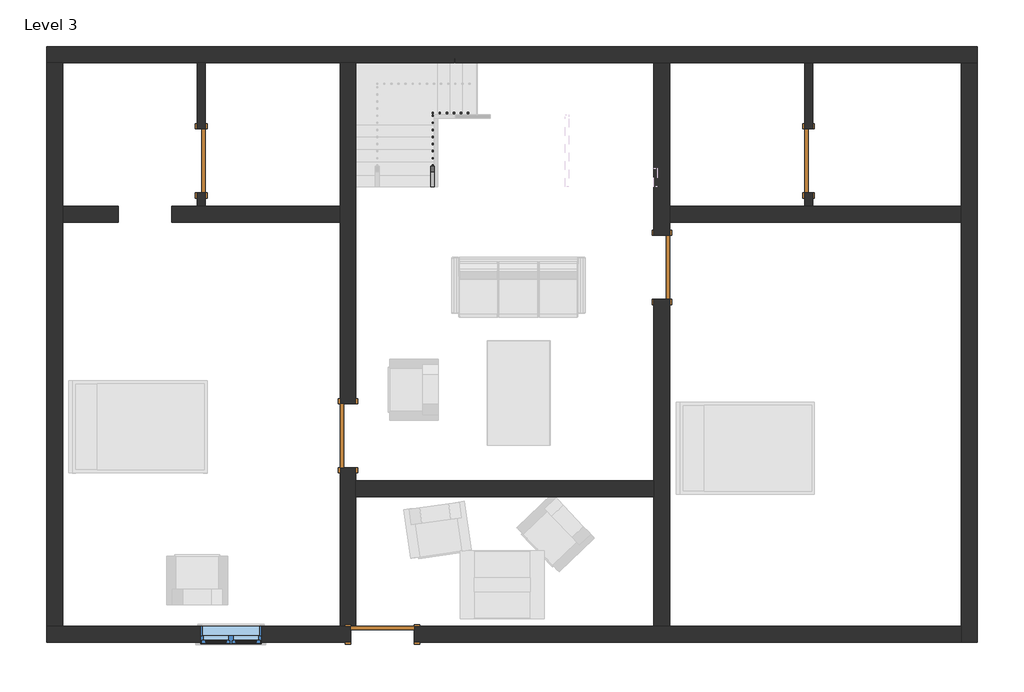
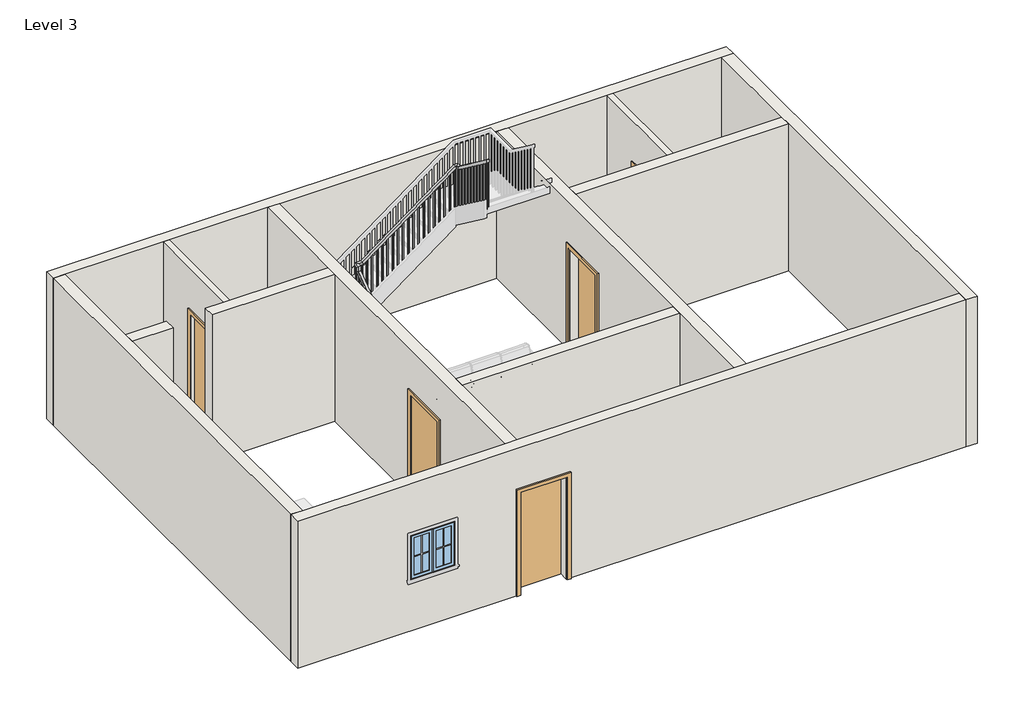
# One storey, part 1 of 2: 12 walls, 5 doors, 1 railing, 1 window.
"""IFC4 building model written with IfcOpenShell, lengths in millimetres."""

from ifc_helpers import new_model, si_unit, frame, origin, place, context, project, spatial, polyline, outline, extrude, faceted_brep, transform, mapped, element, save
from components import door_e5f9f3c4, door_a90ba1ad, door_305aa2a5, window_339605e1

model = new_model("IFC4")

# Units and contexts
model_context = context("Model", 3, world=origin())
ifc_project = project(units=[si_unit("LENGTHUNIT", "METRE", prefix="MILLI")], contexts=[model_context])

# Site, building, storey
site = spatial("IfcSite", under=ifc_project)
building = spatial("IfcBuilding", under=site)
storey = spatial("IfcBuildingStorey", under=building, Name="Level 3", Elevation=3200.4)

# Doors
placement = place(None, origin())
door_shape = door_e5f9f3c4(model_context)
element("IfcDoor", 1, ObjectType="Single-Flush : 36\" x 84\"", at=placement, inside=storey, context=model_context, shape_type="MappedRepresentation", body=[
    mapped(door_shape, transform((-5709.1546642, 5087.2167606, 3200.4), x_axis=(0.0, -1.0, 0.0), y_axis=(1.0, 0.0, 0.0), z_axis=(0.0, 0.0, 1.0))),
])
door_2_shape = door_a90ba1ad(model_context)
element("IfcDoor", 2, ObjectType="Single-Flush : 36\" x 84\"", at=placement, inside=storey, context=model_context, shape_type="MappedRepresentation", body=[
    mapped(door_2_shape, transform((-3607.3046642, 1150.2167606, 3200.4), x_axis=(0.0, -1.0, 0.0), y_axis=(1.0, 0.0, 0.0), z_axis=(0.0, 0.0, 1.0))),
])
element("IfcDoor", 3, ObjectType="Single-Flush : 36\" x 84\"", at=placement, inside=storey, context=model_context, shape_type="MappedRepresentation", body=[
    mapped(door_2_shape, transform((888.4953358, 3563.2167606, 3200.4), x_axis=(0.0, 1.0, 0.0), y_axis=(-1.0, 0.0, 0.0), z_axis=(0.0, 0.0, 1.0))),
])
element("IfcDoor", 4, ObjectType="Single-Flush : 36\" x 84\"", at=placement, inside=storey, context=model_context, shape_type="MappedRepresentation", body=[
    mapped(door_2_shape, transform((-3112.0046642, -1694.5832394, 3200.4), x_axis=(-1.0, 0.0, 0.0), y_axis=(0.0, -1.0, 0.0), z_axis=(0.0, 0.0, 1.0))),
])
door_3_shape = door_305aa2a5(model_context)
element("IfcDoor", 5, ObjectType="Single-Flush : 36\" x 84\"", at=placement, inside=storey, context=model_context, shape_type="MappedRepresentation", body=[
    mapped(door_3_shape, transform((2990.3453358, 5087.2167606, 3200.4), x_axis=(0.0, -1.0, 0.0), y_axis=(1.0, 0.0, 0.0), z_axis=(0.0, 0.0, 1.0))),
])

# Railing
element("IfcRailing", 6, ObjectType="Handrail - Rectangular", at=placement, inside=storey, context=model_context, shape_type="SolidModel", body=[
    faceted_brep([(-2419.4972892, 4718.9167606, 4247.3217391), (-2419.4972892, 4718.9167606, 4183.9634439), (-2368.6972892, 4718.9167606, 4183.9634439), (-2368.6972892, 4718.9167606, 4247.3217391), (-2419.4972892, 5670.3536537, 4956.4672495), (-2419.4972892, 5721.1536537, 4930.9723083), (-2368.6972892, 5721.1536537, 4930.9723083), (-2368.6972892, 5670.3536537, 4956.4672495), (-2419.4972892, 5670.3536537, 5063.2733611), (-2419.4972892, 5721.1536537, 5012.4733611), (-2368.6972892, 5721.1536537, 5012.4733611), (-2368.6972892, 5670.3536537, 5063.2733611), (-2419.4972892, 5797.3536537, 5063.2733611), (-2419.4972892, 5797.3536537, 5012.4733611), (-2368.6972892, 5746.5536537, 5012.4733611), (-2368.6972892, 5746.5536537, 5063.2733611), (-2292.4972892, 5797.3536537, 5063.2733611), (-2275.6482431, 5797.3536537, 5012.4733611), (-2275.6482431, 5746.5536537, 5012.4733611), (-2292.4972892, 5746.5536537, 5063.2733611), (-474.1369697, 5797.3536537, 6418.5729781), (-457.2879235, 5797.3536537, 6367.7729781), (-457.2879235, 5746.5536537, 6367.7729781), (-474.1369697, 5746.5536537, 6418.5729781), (-394.2046642, 5797.3536537, 6418.5729781), (-394.2046642, 5797.3536537, 6367.7729781), (-445.0046642, 5746.5536537, 6367.7729781), (-445.0046642, 5746.5536537, 6418.5729781), (-394.2046642, 5717.4213483, 6418.5729781), (-394.2046642, 5700.5723021, 6367.7729781), (-445.0046642, 5700.5723021, 6367.7729781), (-445.0046642, 5717.4213483, 6418.5729781), (-394.2046642, 4718.9167606, 7162.8), (-445.0046642, 4718.9167606, 7162.8), (-445.0046642, 4718.9167606, 7099.4417047), (-394.2046642, 4718.9167606, 7099.4417047)], [[[0, 1, 2, 3]], [[1, 0, 4, 5]], [[2, 1, 5, 6]], [[3, 2, 6, 7]], [[0, 3, 7, 4]], [[5, 4, 8, 9]], [[6, 5, 9, 10]], [[7, 6, 10, 11]], [[4, 7, 11, 8]], [[9, 8, 12, 13]], [[10, 9, 13, 14]], [[11, 10, 14, 15]], [[8, 11, 15, 12]], [[13, 12, 16, 17]], [[14, 13, 17, 18]], [[15, 14, 18, 19]], [[12, 15, 19, 16]], [[17, 16, 20, 21]], [[18, 17, 21, 22]], [[19, 18, 22, 23]], [[16, 19, 23, 20]], [[21, 20, 24, 25]], [[22, 21, 25, 26]], [[23, 22, 26, 27]], [[20, 23, 27, 24]], [[25, 24, 28, 29]], [[26, 25, 29, 30]], [[27, 26, 30, 31]], [[24, 27, 31, 28]], [[32, 33, 34, 35]], [[29, 28, 32, 35]], [[30, 29, 35, 34]], [[31, 30, 34, 33]], [[28, 31, 33, 32]]]),
    extrude(outline(polyline([(4746.4286537, 7078.9359459), (4765.4786537, 7064.7371882), (4765.4786537, 6115.8782609), (4746.4286537, 6115.8782609), (4746.4286537, 7078.9359459)])), frame((-429.1296642, 0.0, 0.0), z_axis=(1.0, 0.0, 0.0), x_axis=(0.0, 1.0, 0.0)), (0.0, 0.0, 1.0), 19.05),
    extrude(outline(polyline([(4848.0286537, 7003.2092378), (4867.0786537, 6989.0104801), (4867.0786537, 6115.8782609), (4848.0286537, 6115.8782609), (4848.0286537, 7003.2092378)])), frame((-429.1296642, 0.0, 0.0), z_axis=(1.0, 0.0, 0.0), x_axis=(0.0, 1.0, 0.0)), (0.0, 0.0, 1.0), 19.05),
    extrude(outline(polyline([(4949.6286537, 6927.4825298), (4968.6786537, 6913.283772), (4968.6786537, 5983.3565217), (4949.6286537, 5983.3565217), (4949.6286537, 6927.4825298)])), frame((-429.1296642, 0.0, 0.0), z_axis=(1.0, 0.0, 0.0), x_axis=(0.0, 1.0, 0.0)), (0.0, 0.0, 1.0), 19.05),
    extrude(outline(polyline([(5051.2286537, 6851.7558217), (5070.2786537, 6837.5570639), (5070.2786537, 5983.3565217), (5051.2286537, 5983.3565217), (5051.2286537, 6851.7558217)])), frame((-429.1296642, 0.0, 0.0), z_axis=(1.0, 0.0, 0.0), x_axis=(0.0, 1.0, 0.0)), (0.0, 0.0, 1.0), 19.05),
    extrude(outline(polyline([(5152.8286537, 6776.0291136), (5171.8786537, 6761.8303559), (5171.8786537, 5850.8347826), (5152.8286537, 5850.8347826), (5152.8286537, 6776.0291136)])), frame((-429.1296642, 0.0, 0.0), z_axis=(1.0, 0.0, 0.0), x_axis=(0.0, 1.0, 0.0)), (0.0, 0.0, 1.0), 19.05),
    extrude(outline(polyline([(5254.4286537, 6700.3024055), (5273.4786537, 6686.1036478), (5273.4786537, 5718.3130435), (5254.4286537, 5718.3130435), (5254.4286537, 6700.3024055)])), frame((-429.1296642, 0.0, 0.0), z_axis=(1.0, 0.0, 0.0), x_axis=(0.0, 1.0, 0.0)), (0.0, 0.0, 1.0), 19.05),
    extrude(outline(polyline([(5356.0286537, 6624.5756975), (5375.0786537, 6610.3769397), (5375.0786537, 5718.3130435), (5356.0286537, 5718.3130435), (5356.0286537, 6624.5756975)])), frame((-429.1296642, 0.0, 0.0), z_axis=(1.0, 0.0, 0.0), x_axis=(0.0, 1.0, 0.0)), (0.0, 0.0, 1.0), 19.05),
    extrude(outline(polyline([(5457.6286537, 6548.8489894), (5476.6786537, 6534.6502316), (5476.6786537, 5585.7913043), (5457.6286537, 5585.7913043), (5457.6286537, 6548.8489894)])), frame((-429.1296642, 0.0, 0.0), z_axis=(1.0, 0.0, 0.0), x_axis=(0.0, 1.0, 0.0)), (0.0, 0.0, 1.0), 19.05),
    extrude(outline(polyline([(5559.2286537, 6473.1222813), (5578.2786537, 6458.9235236), (5578.2786537, 5585.7913043), (5559.2286537, 5585.7913043), (5559.2286537, 6473.1222813)])), frame((-429.1296642, 0.0, 0.0), z_axis=(1.0, 0.0, 0.0), x_axis=(0.0, 1.0, 0.0)), (0.0, 0.0, 1.0), 19.05),
    extrude(outline(polyline([(5660.8286537, 6397.3955732), (5679.8786537, 6383.1968155), (5679.8786537, 5453.2695652), (5660.8286537, 5453.2695652), (5660.8286537, 6397.3955732)])), frame((-429.1296642, 0.0, 0.0), z_axis=(1.0, 0.0, 0.0), x_axis=(0.0, 1.0, 0.0)), (0.0, 0.0, 1.0), 19.05),
    extrude(outline(polyline([(-473.2222892, 5762.4286537), (-473.2222892, 5781.4786537), (-454.1722892, 5781.4786537), (-454.1722892, 5762.4286537), (-473.2222892, 5762.4286537)])), frame((0.0, 0.0, 5453.2695652), z_axis=(0.0, 0.0, 1.0), x_axis=(1.0, 0.0, 0.0)), (0.0, 0.0, 1.0), 914.5034129),
    extrude(outline(polyline([(6294.3684819, -555.7722892), (6280.1697242, -574.8222892), (5320.7478261, -574.8222892), (5320.7478261, -555.7722892), (6294.3684819, -555.7722892)])), frame((0.0, 5762.4286537, 0.0), z_axis=(0.0, 1.0, 0.0), x_axis=(0.0, 0.0, 1.0)), (0.0, 0.0, 1.0), 19.05),
    extrude(outline(polyline([(6218.6417739, -657.3722892), (6204.4430161, -676.4222892), (5320.7478261, -676.4222892), (5320.7478261, -657.3722892), (6218.6417739, -657.3722892)])), frame((0.0, 5762.4286537, 0.0), z_axis=(0.0, 1.0, 0.0), x_axis=(0.0, 0.0, 1.0)), (0.0, 0.0, 1.0), 19.05),
    extrude(outline(polyline([(6142.9150658, -758.9722892), (6128.716308, -778.0222892), (5188.226087, -778.0222892), (5188.226087, -758.9722892), (6142.9150658, -758.9722892)])), frame((0.0, 5762.4286537, 0.0), z_axis=(0.0, 1.0, 0.0), x_axis=(0.0, 0.0, 1.0)), (0.0, 0.0, 1.0), 19.05),
    extrude(outline(polyline([(6067.1883577, -860.5722892), (6052.9896, -879.6222892), (5188.226087, -879.6222892), (5188.226087, -860.5722892), (6067.1883577, -860.5722892)])), frame((0.0, 5762.4286537, 0.0), z_axis=(0.0, 1.0, 0.0), x_axis=(0.0, 0.0, 1.0)), (0.0, 0.0, 1.0), 19.05),
    extrude(outline(polyline([(5991.4616496, -962.1722892), (5977.2628919, -981.2222892), (5055.7043478, -981.2222892), (5055.7043478, -962.1722892), (5991.4616496, -962.1722892)])), frame((0.0, 5762.4286537, 0.0), z_axis=(0.0, 1.0, 0.0), x_axis=(0.0, 0.0, 1.0)), (0.0, 0.0, 1.0), 19.05),
    extrude(outline(polyline([(5915.7349416, -1063.7722892), (5901.5361838, -1082.8222892), (5055.7043478, -1082.8222892), (5055.7043478, -1063.7722892), (5915.7349416, -1063.7722892)])), frame((0.0, 5762.4286537, 0.0), z_axis=(0.0, 1.0, 0.0), x_axis=(0.0, 0.0, 1.0)), (0.0, 0.0, 1.0), 19.05),
    extrude(outline(polyline([(5840.0082335, -1165.3722892), (5825.8094757, -1184.4222892), (4923.1826087, -1184.4222892), (4923.1826087, -1165.3722892), (5840.0082335, -1165.3722892)])), frame((0.0, 5762.4286537, 0.0), z_axis=(0.0, 1.0, 0.0), x_axis=(0.0, 0.0, 1.0)), (0.0, 0.0, 1.0), 19.05),
    extrude(outline(polyline([(5764.2815254, -1266.9722892), (5750.0827677, -1286.0222892), (4790.6608696, -1286.0222892), (4790.6608696, -1266.9722892), (5764.2815254, -1266.9722892)])), frame((0.0, 5762.4286537, 0.0), z_axis=(0.0, 1.0, 0.0), x_axis=(0.0, 0.0, 1.0)), (0.0, 0.0, 1.0), 19.05),
    extrude(outline(polyline([(5688.5548173, -1368.5722892), (5674.3560596, -1387.6222892), (4790.6608696, -1387.6222892), (4790.6608696, -1368.5722892), (5688.5548173, -1368.5722892)])), frame((0.0, 5762.4286537, 0.0), z_axis=(0.0, 1.0, 0.0), x_axis=(0.0, 0.0, 1.0)), (0.0, 0.0, 1.0), 19.05),
    extrude(outline(polyline([(5612.8281093, -1470.1722892), (5598.6293515, -1489.2222892), (4658.1391304, -1489.2222892), (4658.1391304, -1470.1722892), (5612.8281093, -1470.1722892)])), frame((0.0, 5762.4286537, 0.0), z_axis=(0.0, 1.0, 0.0), x_axis=(0.0, 0.0, 1.0)), (0.0, 0.0, 1.0), 19.05),
    extrude(outline(polyline([(5537.1014012, -1571.7722892), (5522.9026434, -1590.8222892), (4658.1391304, -1590.8222892), (4658.1391304, -1571.7722892), (5537.1014012, -1571.7722892)])), frame((0.0, 5762.4286537, 0.0), z_axis=(0.0, 1.0, 0.0), x_axis=(0.0, 0.0, 1.0)), (0.0, 0.0, 1.0), 19.05),
    extrude(outline(polyline([(5461.3746931, -1673.3722892), (5447.1759354, -1692.4222892), (4525.6173913, -1692.4222892), (4525.6173913, -1673.3722892), (5461.3746931, -1673.3722892)])), frame((0.0, 5762.4286537, 0.0), z_axis=(0.0, 1.0, 0.0), x_axis=(0.0, 0.0, 1.0)), (0.0, 0.0, 1.0), 19.05),
    extrude(outline(polyline([(5385.647985, -1774.9722892), (5371.4492273, -1794.0222892), (4525.6173913, -1794.0222892), (4525.6173913, -1774.9722892), (5385.647985, -1774.9722892)])), frame((0.0, 5762.4286537, 0.0), z_axis=(0.0, 1.0, 0.0), x_axis=(0.0, 0.0, 1.0)), (0.0, 0.0, 1.0), 19.05),
    extrude(outline(polyline([(5309.921277, -1876.5722892), (5295.7225192, -1895.6222892), (4393.0956522, -1895.6222892), (4393.0956522, -1876.5722892), (5309.921277, -1876.5722892)])), frame((0.0, 5762.4286537, 0.0), z_axis=(0.0, 1.0, 0.0), x_axis=(0.0, 0.0, 1.0)), (0.0, 0.0, 1.0), 19.05),
    extrude(outline(polyline([(5234.1945689, -1978.1722892), (5219.9958111, -1997.2222892), (4260.573913, -1997.2222892), (4260.573913, -1978.1722892), (5234.1945689, -1978.1722892)])), frame((0.0, 5762.4286537, 0.0), z_axis=(0.0, 1.0, 0.0), x_axis=(0.0, 0.0, 1.0)), (0.0, 0.0, 1.0), 19.05),
    extrude(outline(polyline([(5158.4678608, -2079.7722892), (5144.2691031, -2098.8222892), (4260.573913, -2098.8222892), (4260.573913, -2079.7722892), (5158.4678608, -2079.7722892)])), frame((0.0, 5762.4286537, 0.0), z_axis=(0.0, 1.0, 0.0), x_axis=(0.0, 0.0, 1.0)), (0.0, 0.0, 1.0), 19.05),
    extrude(outline(polyline([(5082.7411527, -2181.3722892), (5068.542395, -2200.4222892), (4128.0521739, -2200.4222892), (4128.0521739, -2181.3722892), (5082.7411527, -2181.3722892)])), frame((0.0, 5762.4286537, 0.0), z_axis=(0.0, 1.0, 0.0), x_axis=(0.0, 0.0, 1.0)), (0.0, 0.0, 1.0), 19.05),
    extrude(outline(polyline([(5007.0144447, -2282.9722892), (4992.8156869, -2302.0222892), (4128.0521739, -2302.0222892), (4128.0521739, -2282.9722892), (5007.0144447, -2282.9722892)])), frame((0.0, 5762.4286537, 0.0), z_axis=(0.0, 1.0, 0.0), x_axis=(0.0, 0.0, 1.0)), (0.0, 0.0, 1.0), 19.05),
    extrude(outline(polyline([(-2384.5722892, 5725.3917606), (-2403.6222892, 5725.3917606), (-2403.6222892, 5744.4417606), (-2384.5722892, 5744.4417606), (-2384.5722892, 5725.3917606)])), frame((0.0, 0.0, 3995.5304348), z_axis=(0.0, 0.0, 1.0), x_axis=(1.0, 0.0, 0.0)), (0.0, 0.0, 1.0), 1016.9429263),
    extrude(outline(polyline([(5623.7917606, 4858.4044377), (5642.8417606, 4872.6031954), (5642.8417606, 3995.5304348), (5623.7917606, 3995.5304348), (5623.7917606, 4858.4044377)])), frame((-2403.6222892, 0.0, 0.0), z_axis=(1.0, 0.0, 0.0), x_axis=(0.0, 1.0, 0.0)), (0.0, 0.0, 1.0), 19.05),
    extrude(outline(polyline([(5522.1917606, 4782.6777296), (5541.2417606, 4796.8764873), (5541.2417606, 3863.0086957), (5522.1917606, 3863.0086957), (5522.1917606, 4782.6777296)])), frame((-2403.6222892, 0.0, 0.0), z_axis=(1.0, 0.0, 0.0), x_axis=(0.0, 1.0, 0.0)), (0.0, 0.0, 1.0), 19.05),
    extrude(outline(polyline([(5420.5917606, 4706.9510215), (5439.6417606, 4721.1497793), (5439.6417606, 3863.0086957), (5420.5917606, 3863.0086957), (5420.5917606, 4706.9510215)])), frame((-2403.6222892, 0.0, 0.0), z_axis=(1.0, 0.0, 0.0), x_axis=(0.0, 1.0, 0.0)), (0.0, 0.0, 1.0), 19.05),
    extrude(outline(polyline([(5318.9917606, 4631.2243134), (5338.0417606, 4645.4230712), (5338.0417606, 3730.4869565), (5318.9917606, 3730.4869565), (5318.9917606, 4631.2243134)])), frame((-2403.6222892, 0.0, 0.0), z_axis=(1.0, 0.0, 0.0), x_axis=(0.0, 1.0, 0.0)), (0.0, 0.0, 1.0), 19.05),
    extrude(outline(polyline([(5217.3917606, 4555.4976054), (5236.4417606, 4569.6963631), (5236.4417606, 3597.9652174), (5217.3917606, 3597.9652174), (5217.3917606, 4555.4976054)])), frame((-2403.6222892, 0.0, 0.0), z_axis=(1.0, 0.0, 0.0), x_axis=(0.0, 1.0, 0.0)), (0.0, 0.0, 1.0), 19.05),
    extrude(outline(polyline([(5115.7917606, 4479.7708973), (5134.8417606, 4493.969655), (5134.8417606, 3597.9652174), (5115.7917606, 3597.9652174), (5115.7917606, 4479.7708973)])), frame((-2403.6222892, 0.0, 0.0), z_axis=(1.0, 0.0, 0.0), x_axis=(0.0, 1.0, 0.0)), (0.0, 0.0, 1.0), 19.05),
    extrude(outline(polyline([(5014.1917606, 4404.0441892), (5033.2417606, 4418.242947), (5033.2417606, 3465.4434783), (5014.1917606, 3465.4434783), (5014.1917606, 4404.0441892)])), frame((-2403.6222892, 0.0, 0.0), z_axis=(1.0, 0.0, 0.0), x_axis=(0.0, 1.0, 0.0)), (0.0, 0.0, 1.0), 19.05),
    extrude(outline(polyline([(4912.5917606, 4328.3174811), (4931.6417606, 4342.5162389), (4931.6417606, 3465.4434783), (4912.5917606, 3465.4434783), (4912.5917606, 4328.3174811)])), frame((-2403.6222892, 0.0, 0.0), z_axis=(1.0, 0.0, 0.0), x_axis=(0.0, 1.0, 0.0)), (0.0, 0.0, 1.0), 19.05),
    extrude(outline(polyline([(4810.9917606, 4252.5907731), (4830.0417606, 4266.7895308), (4830.0417606, 3332.9217391), (4810.9917606, 3332.9217391), (4810.9917606, 4252.5907731)])), frame((-2403.6222892, 0.0, 0.0), z_axis=(1.0, 0.0, 0.0), x_axis=(0.0, 1.0, 0.0)), (0.0, 0.0, 1.0), 19.05),
    extrude(outline(polyline([(-429.1296642, 5762.4286537), (-429.1296642, 5781.4786537), (-410.0796642, 5781.4786537), (-410.0796642, 5762.4286537), (-429.1296642, 5762.4286537)])), frame((0.0, 0.0, 5453.2695652), z_axis=(0.0, 0.0, 1.0), x_axis=(1.0, 0.0, 0.0)), (0.0, 0.0, 1.0), 914.5034129),
    extrude(outline(polyline([(-2384.5722892, 5762.4286537), (-2403.6222892, 5762.4286537), (-2403.6222892, 5781.4786537), (-2384.5722892, 5781.4786537), (-2384.5722892, 5762.4286537)])), frame((0.0, 0.0, 3995.5304348), z_axis=(0.0, 0.0, 1.0), x_axis=(1.0, 0.0, 0.0)), (0.0, 0.0, 1.0), 1016.9429263),
    extrude(outline(polyline([(4718.9167606, 7099.4417047), (4737.9667606, 7085.242947), (4737.9667606, 6115.8782609), (4718.9167606, 6115.8782609), (4718.9167606, 7099.4417047)])), frame((-429.1296642, 0.0, 0.0), z_axis=(1.0, 0.0, 0.0), x_axis=(0.0, 1.0, 0.0)), (0.0, 0.0, 1.0), 19.05),
    extrude(outline(polyline([(4718.9167606, 4183.9634439), (4737.9667606, 4198.1622016), (4737.9667606, 3332.9217391), (4718.9167606, 3332.9217391), (4718.9167606, 4183.9634439)])), frame((-2403.6222892, 0.0, 0.0), z_axis=(1.0, 0.0, 0.0), x_axis=(0.0, 1.0, 0.0)), (0.0, 0.0, 1.0), 19.05),
])

# Walls
element("IfcWall", 7, ObjectType="WALL4.5\"", at=placement, inside=storey, context=model_context, shape_type="SweptSolid", body=[
    extrude(outline(polyline([(4630.0167606, 5334.0), (4630.0167606, 3200.4), (4439.5167606, 3200.4), (4439.5167606, 6248.4), (6496.9167606, 6248.4), (6496.9167606, 3200.4), (5544.4167606, 3200.4), (5544.4167606, 5334.0), (4630.0167606, 5334.0)])), frame((-5766.3046642, 0.0, 0.0), z_axis=(1.0, 0.0, 0.0), x_axis=(0.0, 1.0, 0.0)), (0.0, 0.0, 1.0), 114.3),
])
element("IfcWall", 8, ObjectType="WALL4.5\"", at=placement, inside=storey, context=model_context, shape_type="SweptSolid", body=[
    extrude(outline(polyline([(4630.0167606, 5334.0), (4630.0167606, 3200.4), (4439.5167606, 3200.4), (4439.5167606, 6248.4), (6496.9167606, 6248.4), (6496.9167606, 3200.4), (5544.4167606, 3200.4), (5544.4167606, 5334.0), (4630.0167606, 5334.0)])), frame((2933.1953358, 0.0, 0.0), z_axis=(1.0, 0.0, 0.0), x_axis=(0.0, 1.0, 0.0)), (0.0, 0.0, 1.0), 114.3),
])
element("IfcWall", 9, ObjectType="WALL9\"", at=placement, inside=storey, context=model_context, shape_type="Brep", body=[
    faceted_brep([(-7925.3046642, 6496.9167606, 3200.4), (-7696.7046642, 6496.9167606, 3200.4), (-5766.3046642, 6496.9167606, 3200.4), (-5652.0046642, 6496.9167606, 3200.4), (-3721.6046642, 6496.9167606, 3200.4), (-3493.0046642, 6496.9167606, 3200.4), (774.1953358, 6496.9167606, 3200.4), (1002.7953358, 6496.9167606, 3200.4), (2933.1953358, 6496.9167606, 3200.4), (3047.4953358, 6496.9167606, 3200.4), (5181.0953358, 6496.9167606, 3200.4), (5409.6953358, 6496.9167606, 3200.4), (5409.6953358, 6496.9167606, 6248.4), (5181.0953358, 6496.9167606, 6248.4), (3047.4953358, 6496.9167606, 6248.4), (2933.1953358, 6496.9167606, 6248.4), (1002.7953358, 6496.9167606, 6248.4), (774.1953358, 6496.9167606, 6248.4), (-3493.0046642, 6496.9167606, 6248.4), (-3721.6046642, 6496.9167606, 6248.4), (-5652.0046642, 6496.9167606, 6248.4), (-5766.3046642, 6496.9167606, 6248.4), (-7696.7046642, 6496.9167606, 6248.4), (-7925.3046642, 6496.9167606, 6248.4), (-7925.3046642, 6725.5167606, 3200.4), (-7925.3046642, 6725.5167606, 6248.4), (5409.6953358, 6725.5167606, 6248.4), (5409.6953358, 6725.5167606, 3200.4)], [[[0, 1, 2, 3, 4, 5, 6, 7, 8, 9, 10, 11, 12, 13, 14, 15, 16, 17, 18, 19, 20, 21, 22, 23]], [[24, 25, 26, 27]], [[11, 10, 9, 8, 7, 6, 5, 4, 3, 2, 1, 0, 24, 27]], [[12, 11, 27, 26]], [[0, 23, 25, 24]], [[23, 22, 21, 20, 19, 18, 17, 16, 15, 14, 13, 12, 26, 25]]]),
])
element("IfcWall", 10, ObjectType="WALL9\"", at=placement, inside=storey, context=model_context, shape_type="Brep", body=[
    faceted_brep([(5181.0953358, 6496.9167606, 3200.4), (5181.0953358, 4439.5167606, 3200.4), (5181.0953358, 4210.9167606, 3200.4), (5181.0953358, -1580.2832394, 3200.4), (5181.0953358, -1808.8832394, 3200.4), (5181.0953358, -1808.8832394, 6248.4), (5181.0953358, -1580.2832394, 6248.4), (5181.0953358, 4210.9167606, 6248.4), (5181.0953358, 4439.5167606, 6248.4), (5181.0953358, 6496.9167606, 6248.4), (5409.6953358, 6496.9167606, 3200.4), (5409.6953358, 6496.9167606, 6248.4), (5409.6953358, -1808.8832394, 6248.4), (5409.6953358, -1808.8832394, 3200.4)], [[[0, 1, 2, 3, 4, 5, 6, 7, 8, 9]], [[10, 11, 12, 13]], [[4, 3, 2, 1, 0, 10, 13]], [[0, 9, 11, 10]], [[5, 4, 13, 12]], [[9, 8, 7, 6, 5, 12, 11]]]),
])
element("IfcWall", 11, ObjectType="WALL9\"", at=placement, inside=storey, context=model_context, shape_type="Brep", body=[
    faceted_brep([(-3569.2046642, -1580.2832394, 5334.0), (-3569.2046642, -1580.2832394, 3200.4), (-3721.6046642, -1580.2832394, 3200.4), (-7696.7046642, -1580.2832394, 3200.4), (-7925.3046642, -1580.2832394, 3200.4), (-7925.3046642, -1580.2832394, 6248.4), (-7696.7046642, -1580.2832394, 6248.4), (-3721.6046642, -1580.2832394, 6248.4), (-3493.0046642, -1580.2832394, 6248.4), (774.1953358, -1580.2832394, 6248.4), (1002.7953358, -1580.2832394, 6248.4), (5181.0953358, -1580.2832394, 6248.4), (5181.0953358, -1580.2832394, 3200.4), (1002.7953358, -1580.2832394, 3200.4), (774.1953358, -1580.2832394, 3200.4), (-2654.8046642, -1580.2832394, 3200.4), (-2654.8046642, -1580.2832394, 5334.0), (-5715.5046642, -1580.2832394, 5181.9434313), (-5715.5046642, -1580.2832394, 4267.5434313), (-4851.9046642, -1580.2832394, 4267.5434313), (-4851.9046642, -1580.2832394, 5181.9434313), (-7925.3046642, -1808.8832394, 3200.4), (-3569.2046642, -1808.8832394, 3200.4), (-3569.2046642, -1808.8832394, 5334.0), (-2654.8046642, -1808.8832394, 5334.0), (-2654.8046642, -1808.8832394, 3200.4), (5181.0953358, -1808.8832394, 3200.4), (5181.0953358, -1808.8832394, 6248.4), (-7925.3046642, -1808.8832394, 6248.4), (-5715.5046642, -1808.8832394, 5181.9434313), (-4851.9046642, -1808.8832394, 5181.9434313), (-4851.9046642, -1808.8832394, 4267.5434313), (-5715.5046642, -1808.8832394, 4267.5434313)], [[[0, 1, 2, 3, 4, 5, 6, 7, 8, 9, 10, 11, 12, 13, 14, 15, 16], [17, 18, 19, 20]], [[21, 22, 23, 24, 25, 26, 27, 28], [29, 30, 31, 32]], [[4, 3, 2, 1, 22, 21]], [[15, 14, 13, 12, 26, 25]], [[12, 11, 27, 26]], [[5, 4, 21, 28]], [[23, 22, 1, 0]], [[24, 23, 0, 16]], [[25, 24, 16, 15]], [[11, 10, 9, 8, 7, 6, 5, 28, 27]], [[18, 17, 29, 32]], [[19, 18, 32, 31]], [[20, 19, 31, 30]], [[17, 20, 30, 29]]]),
])
element("IfcWall", 12, ObjectType="WALL9\"", at=placement, inside=storey, context=model_context, shape_type="Brep", body=[
    faceted_brep([(-7696.7046642, -1580.2832394, 3200.4), (-7696.7046642, 4210.9167606, 3200.4), (-7696.7046642, 4439.5167606, 3200.4), (-7696.7046642, 6496.9167606, 3200.4), (-7696.7046642, 6496.9167606, 6248.4), (-7696.7046642, 4439.5167606, 6248.4), (-7696.7046642, 4210.9167606, 6248.4), (-7696.7046642, -1580.2832394, 6248.4), (-7925.3046642, -1580.2832394, 3200.4), (-7925.3046642, -1580.2832394, 6248.4), (-7925.3046642, 6496.9167606, 6248.4), (-7925.3046642, 6496.9167606, 3200.4)], [[[0, 1, 2, 3, 4, 5, 6, 7]], [[8, 9, 10, 11]], [[3, 2, 1, 0, 8, 11]], [[4, 3, 11, 10]], [[0, 7, 9, 8]], [[7, 6, 5, 4, 10, 9]]]),
])
element("IfcWall", 13, ObjectType="WALL9\"", at=placement, inside=storey, context=model_context, shape_type="Brep", body=[
    faceted_brep([(-3721.6046642, 693.0167606, 5334.0), (-3721.6046642, 693.0167606, 3200.4), (-3721.6046642, -1580.2832394, 3200.4), (-3721.6046642, -1580.2832394, 6248.4), (-3721.6046642, 4210.9167606, 6248.4), (-3721.6046642, 4439.5167606, 6248.4), (-3721.6046642, 6496.9167606, 6248.4), (-3721.6046642, 6496.9167606, 3200.4), (-3721.6046642, 4439.5167606, 3200.4), (-3721.6046642, 4210.9167606, 3200.4), (-3721.6046642, 1607.4167606, 3200.4), (-3721.6046642, 1607.4167606, 5334.0), (-3493.0046642, -1580.2832394, 3200.4), (-3493.0046642, 273.9167606, 3200.4), (-3493.0046642, 502.5167606, 3200.4), (-3493.0046642, 693.0167606, 3200.4), (-3493.0046642, 693.0167606, 5334.0), (-3493.0046642, 1607.4167606, 5334.0), (-3493.0046642, 1607.4167606, 3200.4), (-3493.0046642, 6496.9167606, 3200.4), (-3493.0046642, 6496.9167606, 6248.4), (-3493.0046642, 502.5167606, 6248.4), (-3493.0046642, 273.9167606, 6248.4), (-3493.0046642, -1580.2832394, 6248.4), (-3569.2046642, -1580.2832394, 3200.4)], [[[0, 1, 2, 3, 4, 5, 6, 7, 8, 9, 10, 11]], [[12, 13, 14, 15, 16, 17, 18, 19, 20, 21, 22, 23]], [[2, 1, 15, 14, 13, 12, 24]], [[10, 9, 8, 7, 19, 18]], [[7, 6, 20, 19]], [[3, 2, 24, 12, 23]], [[16, 15, 1, 0]], [[17, 16, 0, 11]], [[18, 17, 11, 10]], [[6, 5, 4, 3, 23, 22, 21, 20]]]),
])
element("IfcWall", 14, ObjectType="WALL9\"", at=placement, inside=storey, context=model_context, shape_type="Brep", body=[
    faceted_brep([(774.1953358, 6496.9167606, 3200.4), (774.1953358, 4020.4167606, 3200.4), (774.1953358, 4020.4167606, 5334.0), (774.1953358, 3106.0167606, 5334.0), (774.1953358, 3106.0167606, 3200.4), (774.1953358, 502.5167606, 3200.4), (774.1953358, 273.9167606, 3200.4), (774.1953358, -1580.2832394, 3200.4), (774.1953358, -1580.2832394, 6248.4), (774.1953358, 273.9167606, 6248.4), (774.1953358, 502.5167606, 6248.4), (774.1953358, 4668.1167606, 6248.4), (774.1953358, 6446.1167606, 6248.4), (774.1953358, 6496.9167606, 6248.4), (1002.7953358, 4020.4167606, 5334.0), (1002.7953358, 4020.4167606, 3200.4), (1002.7953358, 4210.9167606, 3200.4), (1002.7953358, 4439.5167606, 3200.4), (1002.7953358, 6496.9167606, 3200.4), (1002.7953358, 6496.9167606, 6248.4), (1002.7953358, 4439.5167606, 6248.4), (1002.7953358, 4210.9167606, 6248.4), (1002.7953358, -1580.2832394, 6248.4), (1002.7953358, -1580.2832394, 3200.4), (1002.7953358, 3106.0167606, 3200.4), (1002.7953358, 3106.0167606, 5334.0)], [[[0, 1, 2, 3, 4, 5, 6, 7, 8, 9, 10, 11, 12, 13]], [[14, 15, 16, 17, 18, 19, 20, 21, 22, 23, 24, 25]], [[24, 23, 7, 6, 5, 4]], [[18, 17, 16, 15, 1, 0]], [[0, 13, 19, 18]], [[8, 7, 23, 22]], [[2, 1, 15, 14]], [[3, 2, 14, 25]], [[4, 3, 25, 24]], [[13, 12, 11, 10, 9, 8, 22, 21, 20, 19]]]),
])
element("IfcWall", 15, ObjectType="WALL9\"", at=placement, inside=storey, context=model_context, shape_type="SweptSolid", body=[
    extrude(outline(polyline([(774.1953358, 273.9167606), (-3493.0046642, 273.9167606), (-3493.0046642, 502.5167606), (774.1953358, 502.5167606), (774.1953358, 273.9167606)])), frame((0.0, 0.0, 3200.4), z_axis=(0.0, 0.0, 1.0), x_axis=(1.0, 0.0, 0.0)), (0.0, 0.0, 1.0), 3048.0),
])
element("IfcWall", 16, ObjectType="WALL9\"", at=placement, inside=storey, context=model_context, shape_type="SweptSolid", body=[
    extrude(outline(polyline([(-6895.4507894, 4210.9167606), (-7696.7046642, 4210.9167606), (-7696.7046642, 4439.5167606), (-6895.4507894, 4439.5167606), (-6895.4507894, 4210.9167606)])), frame((0.0, 0.0, 3200.4), z_axis=(0.0, 0.0, 1.0), x_axis=(1.0, 0.0, 0.0)), (0.0, 0.0, 1.0), 3048.0),
])
element("IfcWall", 17, ObjectType="WALL9\"", at=placement, inside=storey, context=model_context, shape_type="Brep", body=[
    faceted_brep([(-3721.6046642, 4439.5167606, 3200.4), (-5652.0046642, 4439.5167606, 3200.4), (-5766.3046642, 4439.5167606, 3200.4), (-6131.0963491, 4439.5167606, 3200.4), (-6131.0963491, 4439.5167606, 6248.4), (-5766.3046642, 4439.5167606, 6248.4), (-5652.0046642, 4439.5167606, 6248.4), (-3721.6046642, 4439.5167606, 6248.4), (-3721.6046642, 4210.9167606, 3200.4), (-3721.6046642, 4210.9167606, 6248.4), (-6131.0963491, 4210.9167606, 6248.4), (-6131.0963491, 4210.9167606, 3200.4)], [[[0, 1, 2, 3, 4, 5, 6, 7]], [[8, 9, 10, 11]], [[3, 2, 1, 0, 8, 11]], [[4, 3, 11, 10]], [[0, 7, 9, 8]], [[7, 6, 5, 4, 10, 9]]]),
])
element("IfcWall", 18, ObjectType="WALL9\"", at=placement, inside=storey, context=model_context, shape_type="Brep", body=[
    faceted_brep([(1002.7953358, 4210.9167606, 3200.4), (5181.0953358, 4210.9167606, 3200.4), (5181.0953358, 4210.9167606, 6248.4), (1002.7953358, 4210.9167606, 6248.4), (1002.7953358, 4439.5167606, 3200.4), (1002.7953358, 4439.5167606, 6248.4), (2933.1953358, 4439.5167606, 6248.4), (3047.4953358, 4439.5167606, 6248.4), (5181.0953358, 4439.5167606, 6248.4), (5181.0953358, 4439.5167606, 3200.4), (3047.4953358, 4439.5167606, 3200.4), (2933.1953358, 4439.5167606, 3200.4)], [[[0, 1, 2, 3]], [[4, 5, 6, 7, 8, 9, 10, 11]], [[1, 0, 4, 11, 10, 9]], [[2, 1, 9, 8]], [[0, 3, 5, 4]], [[3, 2, 8, 7, 6, 5]]]),
])

# Window
window_shape = window_339605e1(model_context)
element("IfcWindow", 19, ObjectType="Window-Casement-Double : 34\" x 36\"", at=placement, inside=storey, context=model_context, shape_type="MappedRepresentation", body=[
    mapped(window_shape, transform((-5283.7046642, -1694.5832394, 3353.1434313), x_axis=(-1.0, 0.0, 0.0), y_axis=(0.0, -1.0, 0.0), z_axis=(0.0, 0.0, 1.0))),
])

save(model, "model.ifc")

# Revit data of these elements
# Type "Single-Flush : 36\" x 84\""
#   Type Mark = "1"
#   Construction Type Id = "MDOOR"
#   Assembly Code = "C1020"
#   Analytic Construction = "Metal"
#   Thickness = 0' - 2"
#   Heat Transfer Coefficient (U) = 0.651978 BTU/(h·ft²·°F)
#   Height = 7' - 0"
#   Trim Projection Ext = 0' - 1"
#   Trim Projection Int = 0' - 1"
#   Trim Width = 0' - 3"
#   Width = 3' - 0"
#   Define Thermal Properties by = 1
#   Define Thermal Properties by = 1
#   Door Material = Door - Panel
#   Frame Material = Door - Frame
#   Visual Light Transmittance = 0
#   Solar Heat Gain Coefficient = 0
#   Function = (empty or 0)
#   Wall Closure = (empty or 0)
# Type "Handrail - Rectangular"
#   Assembly Code = "C2010400"
#   built-in parameter 1008612 = 0.0416667 (stored number, unit not read)
#   built-in parameter 1008611 = 0.0416667 (stored number, unit not read)
#   built-in parameter 1008609 = 0.333333 (stored number, unit not read)
#   built-in parameter 1008604 = 0.166667 (stored number, unit not read)
#   built-in parameter 1008603 = 0.166667 (stored number, unit not read)
#   Railing Height = 3' - 0"
#   built-in parameter 1008630 = 2
#   built-in parameter 1008610 = 2
#   built-in parameter 1008618 = Baluster - Square : 3/4"
# Type "WALL4.5\""
#   Assembly Code = "B2010"
#   Layers, outside or top first: 0' - 4 1/2" no material (function 1)
# Type "WALL9\""
#   Assembly Code = "B2010"
#   Layers, outside or top first: 0' - 9" no material (function 1)
# Type "Window-Casement-Double : 34\" x 36\""
#   Type Mark = "14"
#   Fire Rating = "0.5h"
#   Assembly Code = "B2020100"
#   Analytic Construction = "Double glazing - domestic"
#   Frame Extension [instance default] = 0' - 0 1/4"
#   Window Inset [instance default] = 0' - 0"
#   Wall Thickness [instance default] = 0' - 6"
#   Interior Wall Closure [instance default] = 0' - 2 1/4"
#   Half Width = 1' - 5"
#   Visual Light Transmittance = 0.81
#   Thermal Resistance (R) = 1.8146 (h·ft²·°F)/BTU
#   Solar Heat Gain Coefficient = 0.76
#   Rough Width = 2' - 10 1/2"
#   Rough Height = 3' - 0 1/2"
#   Height = 3' - 0"
#   Heat Transfer Coefficient (U) = 0.5511 BTU/(h·ft²·°F)
#   Exterior Wall Closure [instance default] = 0' - 1 1/4"
#   Extension Jamb [instance default] = 0' - 2 1/4"
#   Default Sill Height = 3' - 0"
#   Width = 2' - 10"
#   Define Thermal Properties by = 0
#   Muntin Visibility = yes
#   Interior Trim Visibility [instance default] = yes
#   Exterior Trim Visibility [instance default] = yes
#   Extension Jamb Visibility [instance default] = yes
#   Interior Trim Material = Wood - Stained
#   Muntin Pattern = Muntin Pattern_2x2 : Muntin Pattern_2x2
#   Interior Trim = Trim-Window-Interior-Flat : Picture Frame
#   Interior Frame Material = Wood - Stained
#   Glass Panel Material = Glass
#   Exterior Trim Material = Clad - White
#   Exterior Trim = Trim-Window-Exterior-Flat : with Sill
#   Exterior Frame Material = Clad - White
#   Wall Closure = (empty or 0)
# Elements 1, 2, 3, 4, 5 (IfcDoor, "Single-Flush : 36\" x 84\"")
#   Phase Created = New Construction
#   Materials on its faces: "Door - Frame", "Door - Panel"
# Element 6 (IfcRailing, "Handrail - Rectangular")
#   Phase Created = New Construction
# Elements 7, 8 (IfcWall, "WALL4.5\"")
#   Top Offset = 0' - 0"
#   Base Offset = 0' - 0"
#   Unconnected Height = 10' - 0"
#   wall height = 10' - 0"
#   Phase Created = New Construction
#   Base Constraint = Level 3
#   Materials on its faces: "Default Wall"
# Elements 9, 10, 11, 12, 13, 14, 15, 16, 17, 18 (IfcWall, "WALL9\"")
#   Top Offset = 0' - 0"
#   Base Offset = 0' - 0"
#   Unconnected Height = 10' - 0"
#   wall height = 10' - 0"
#   Phase Created = New Construction
#   Base Constraint = Level 3
#   Materials on its faces: "Default Wall"
# Element 19 (IfcWindow, "Window-Casement-Double : 34\" x 36\"")
#   Mark = "2"
#   Window Inset = 0' - 0"
#   Interior Wall Closure = 0' - 2 1/4"
#   Frame Extension = 0' - 0 1/4"
#   Exterior Wall Closure = 0' - 1 1/4"
#   Interior Trim Visibility = yes
#   Exterior Trim Visibility = yes
#   Phase Created = New Construction
#   Materials on its faces: "Wood - Stained", "Glass", "Clad - White"
# Materials
#   "Door - Panel": class "Wood", colour RGB 210 159 95, transparency 0, Cost = 0
#   "Door - Frame": colour RGB 118 70 51, transparency 0, Cost = 0
#   "Wood - Stained": class "Wood", colour RGB 224 178 126, transparency 0, Cost = 0
#   "Glass": class "Glass", colour RGB 0 128 192, transparency 0.75, Description = "Soda Lime Glass", Cost = 0
#   "Clad - White": class "Wood", colour RGB 242 242 238, transparency 0, Cost = 0
#   "Default Wall": colour RGB 128 128 128, transparency 0, Cost = 0
